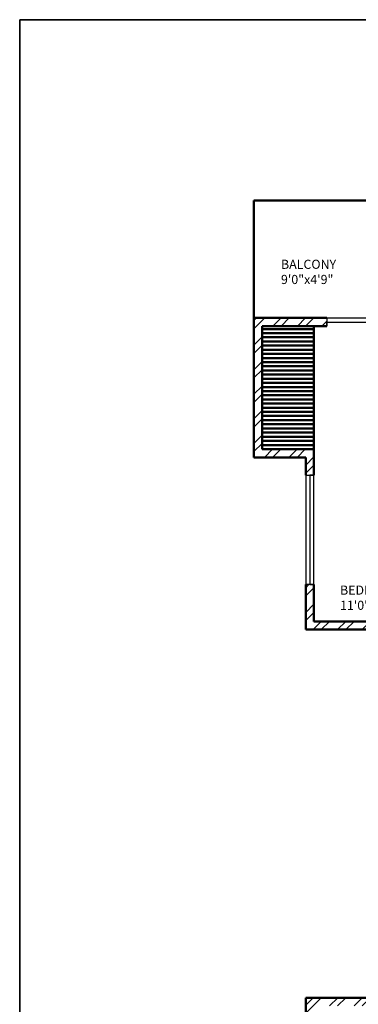
# Model space of a CAD drawing. Units: inches. Extents: x 963 to 2075, y 289 to 2657.
# Tile 59 of 98: x 963 to 1149, y 2117 to 2657. Entities that reach past the tile are written whole.
import ezdxf

# ---------------------------------------------------------------- set-up
doc = ezdxf.new("R2010")
doc.units = ezdxf.units.IN
for name, color, linetype, lineweight in [('A-ANNO-TTLB', 7, 'Continuous', 35), ('A-AREA-IDEN', 7, 'Continuous', 18), ('A-GLAZ', 3, 'Continuous', 25), ('A-WALL', 7, 'Continuous', 50), ('A-WALL-PATT', 8, 'Continuous', 13)]:
    doc.layers.add(name, color=color, linetype=linetype, lineweight=lineweight)
doc.styles.get("Standard").update_dxf_attribs({"font": 'arial.ttf'})

msp = doc.modelspace()

# ---------------------------------------------------------------- hatches: boundary and pattern name
at = {"layer": 'A-WALL-PATT'}
h = msp.add_hatch(dxfattribs=at)
h.set_pattern_fill('ANSI32', color=256)
h.paths.add_polyline_path([(1296.92, 2558.32), (1203.92, 2558.32), (1203.92, 2493.82), (1191.53, 2493.82), (1191.53, 2489.32), (1211.06, 2489.32), (1211.06, 2492.02), (1211.06, 2493.82), (1208.42, 2493.82), (1208.42, 2553.82), (1292.42, 2553.82), (1292.42, 2538.86), (1296.92, 2538.86)])
h.paths.add_polyline_path([(1442.42, 2558.32), (1349.42, 2558.32), (1349.42, 2538.94), (1353.92, 2538.94), (1353.92, 2553.82), (1437.92, 2553.82), (1437.92, 2493.82), (1434.54, 2493.82), (1434.54, 2489.32), (1448.31, 2489.32), (1448.31, 2491.57), (1448.31, 2493.82), (1442.42, 2493.82)])
h.paths.add_polyline_path([(1415.55, 2491.57), (1415.55, 2493.82), (1340.94, 2493.82), (1340.94, 2489.32), (1371.92, 2489.32), (1371.92, 2378.32), (1367.6, 2378.32), (1367.6, 2373.82), (1371.92, 2373.82), (1371.92, 2355.19), (1376.42, 2355.19), (1376.42, 2489.32), (1415.55, 2489.32)])
h.paths.add_polyline_path([(1304.94, 2491.57), (1304.94, 2493.82), (1296.92, 2493.82), (1296.92, 2514.86), (1292.42, 2514.86), (1292.42, 2493.82), (1232.81, 2493.82), (1232.81, 2489.32), (1256.42, 2489.32), (1256.42, 2327.32), (1253.71, 2327.32), (1253.71, 2322.82), (1328.42, 2322.82), (1328.42, 2331.15), (1323.92, 2331.15), (1323.92, 2327.32), (1260.92, 2327.32), (1260.92, 2373.82), (1323.92, 2373.82), (1323.92, 2357.81), (1328.42, 2357.81), (1328.42, 2373.82), (1346.01, 2373.82), (1346.01, 2376.07), (1346.01, 2378.32), (1260.92, 2378.32), (1260.92, 2489.32), (1304.94, 2489.32)])
h.paths.add_polyline_path([(1226.65, 2327.32), (1124.42, 2327.32), (1124.42, 2347.45), (1119.92, 2347.45), (1119.92, 2322.82), (1163.42, 2322.82), (1163.42, 2305.43), (1165.67, 2305.43), (1167.92, 2305.43), (1167.92, 2322.82), (1226.65, 2322.82), (1226.65, 2325.07)])
h.paths.add_polyline_path([(1095.92, 2489.32), (1124.42, 2489.32), (1131.53, 2489.32), (1131.53, 2491.57), (1131.53, 2493.82), (1119.92, 2493.82), (1091.42, 2493.82), (1091.42, 2417.32), (1095.92, 2417.32), (1119.92, 2417.32), (1119.92, 2407.45), (1124.42, 2407.45), (1124.42, 2421.82), (1095.92, 2421.82)])
h.paths.add_polyline_path([(1512.92, 2558.32), (1508.42, 2558.32), (1508.42, 2493.82), (1503.4, 2493.82), (1503.4, 2489.32), (1508.42, 2489.32), (1508.42, 2327.32), (1376.42, 2327.32), (1376.42, 2330.27), (1371.92, 2330.27), (1371.92, 2298.74), (1376.42, 2298.74), (1376.42, 2322.82), (1508.42, 2322.82), (1508.42, 2165.32), (1504.26, 2165.32), (1504.26, 2160.82), (1508.42, 2160.82), (1508.42, 2108.32), (1512.92, 2108.32), (1512.92, 2160.82), (1516.18, 2160.82), (1516.18, 2163.07), (1516.18, 2165.32), (1512.92, 2165.32), (1512.92, 2322.82), (1644.92, 2322.82), (1644.92, 2298.74), (1649.42, 2298.74), (1649.42, 2322.82), (1649.42, 2330.94), (1647.17, 2330.94), (1644.92, 2330.94), (1644.92, 2327.32), (1512.92, 2327.32), (1512.92, 2489.32), (1516.76, 2489.32), (1516.76, 2491.57), (1516.76, 2493.82), (1512.92, 2493.82)])
h.paths.add_polyline_path([(1671.92, 2558.32), (1578.92, 2558.32), (1578.92, 2493.82), (1573.53, 2493.82), (1573.53, 2489.32), (1586.54, 2489.32), (1586.54, 2491.57), (1586.54, 2493.82), (1583.42, 2493.82), (1583.42, 2553.82), (1667.42, 2553.82), (1667.42, 2541.11), (1671.92, 2541.11)])
h.paths.add_polyline_path([(1681.26, 2493.82), (1671.92, 2493.82), (1671.92, 2517.11), (1667.42, 2517.11), (1667.42, 2493.82), (1610.22, 2493.82), (1610.22, 2489.32), (1644.92, 2489.32), (1644.92, 2357.87), (1649.42, 2357.87), (1649.42, 2373.82), (1652.2, 2373.82), (1652.2, 2375.83), (1652.2, 2378.32), (1649.42, 2378.32), (1649.42, 2489.32), (1681.26, 2489.32), (1681.26, 2491.57)])
h.paths.add_polyline_path([(1821.92, 2558.32), (1728.92, 2558.32), (1728.92, 2541), (1733.42, 2541), (1733.42, 2553.82), (1817.42, 2553.82), (1817.42, 2493.82), (1813.51, 2493.82), (1813.51, 2489.32), (1830.08, 2489.32), (1830.08, 2491.57), (1830.08, 2493.82), (1821.92, 2493.82)])
h.paths.add_polyline_path([(1794.24, 2493.82), (1717.26, 2493.82), (1717.26, 2489.32), (1760.42, 2489.32), (1760.42, 2378.32), (1674.4, 2378.32), (1674.4, 2373.82), (1692.92, 2373.82), (1692.92, 2356.95), (1697.42, 2356.95), (1697.42, 2373.82), (1760.42, 2373.82), (1760.42, 2327.32), (1697.42, 2327.32), (1697.42, 2333.34), (1692.92, 2333.34), (1692.92, 2322.82), (1768.04, 2322.82), (1768.04, 2325.07), (1768.04, 2327.32), (1764.92, 2327.32), (1764.92, 2489.32), (1794.24, 2489.32)])
h.paths.add_polyline_path([(1733.42, 2517), (1728.92, 2517), (1728.92, 2493.82), (1733.42, 2493.82)], flags=17)
h.paths.add_polyline_path([(1929.92, 2493.82), (1890.08, 2493.82), (1890.08, 2489.32), (1896.92, 2489.32), (1925.42, 2489.32), (1925.42, 2421.82), (1896.92, 2421.82), (1896.92, 2408.32), (1901.42, 2408.32), (1901.42, 2417.32), (1925.42, 2417.32), (1929.92, 2417.32)])
h.paths.add_polyline_path([(1901.42, 2348.32), (1896.92, 2348.32), (1896.92, 2327.32), (1800.42, 2327.32), (1800.42, 2322.82), (1853.42, 2322.82), (1853.42, 2309.45), (1857.92, 2309.45), (1857.92, 2322.82), (1901.42, 2322.82)])
h.paths.add_polyline_path([(1857.92, 2249.45), (1853.42, 2249.45), (1853.42, 2214.82), (1686.31, 2214.82), (1686.31, 2210.32), (1853.42, 2210.32), (1853.42, 2202.13), (1857.92, 2202.13), (1857.92, 2210.32)])
h.paths.add_polyline_path([(1857.92, 2142.13), (1853.42, 2142.13), (1853.42, 2115.42), (1841.42, 2115.42), (1841.42, 2088.53), (1841.42, 2046.95), (1845.92, 2046.95), (1845.92, 2110.92), (1905.92, 2110.92), (1905.92, 2092.52), (1910.42, 2092.52), (1910.42, 2115.42), (1857.92, 2115.42)])
h.paths.add_polyline_path([(1532.44, 1482.34), (1573.46, 1482.34), (1573.46, 1501), (1532.44, 1501)], flags=9)
h.paths.add_polyline_path([(1438.66, 1486.3), (1479.68, 1486.3), (1479.68, 1504.96), (1438.66, 1504.96)], flags=9)
h.paths.add_polyline_path([(1411.22, 1365.31), (1659.14, 1365.31), (1659.14, 1402.4), (1411.22, 1402.4)], flags=9)
h.paths.add_polyline_path([(1185.67, 2296.3), (1248.16, 2296.3), (1248.16, 2314.95), (1185.67, 2314.95)], flags=9)
h.paths.add_polyline_path([(1177.31, 2187.35), (1216.15, 2187.35), (1216.15, 2206.01), (1177.31, 2206.01)], flags=9)
h.paths.add_polyline_path([(1295.1, 1602.08), (1328.26, 1602.08), (1328.26, 1620.74), (1295.1, 1620.74)], flags=9)
h.paths.add_polyline_path([(1525.13, 2005.99), (1558.39, 2005.99), (1558.39, 2024.65), (1525.13, 2024.65)], flags=9)
h.paths.add_polyline_path([(1459.61, 1977.13), (1472.19, 1977.13), (1472.19, 1987.43), (1459.61, 1987.43)], flags=9)
h.paths.add_polyline_path([(1467.81, 2053.68), (1480.02, 2053.68), (1480.02, 2063.98), (1467.81, 2063.98)], flags=9)
h.paths.add_polyline_path([(1555.18, 2119.02), (1584.56, 2119.02), (1584.56, 2137.68), (1555.18, 2137.68)], flags=25)
h.paths.add_polyline_path([(1405.39, 2115.29), (1444.48, 2115.29), (1444.48, 2133.95), (1405.39, 2133.95)], flags=25)
h.paths.add_polyline_path([(1698.48, 2004.26), (1727.69, 2004.26), (1727.69, 2022.92), (1698.48, 2022.92)], flags=9)
h.paths.add_polyline_path([(1612.16, 1972.86), (1629.02, 1972.86), (1629.02, 1983.16), (1612.16, 1983.16)], flags=9)
h.paths.add_polyline_path([(1608.29, 2060.04), (1625.15, 2060.04), (1625.15, 2070.34), (1608.29, 2070.34)], flags=9)
h.paths.add_polyline_path([(1527.95, 1684.4), (1566.79, 1684.4), (1566.79, 1703.06), (1527.95, 1703.06)], flags=9)
h.paths.add_polyline_path([(1422.79, 1683.59), (1461.63, 1683.59), (1461.63, 1702.25), (1422.79, 1702.25)], flags=9)
h.paths.add_polyline_path([(1531.26, 1732.46), (1574.01, 1732.46), (1574.01, 1751.12), (1531.26, 1751.12)], flags=9)
h.paths.add_polyline_path([(1402.87, 1732.85), (1439.8, 1732.85), (1439.8, 1751.5), (1402.87, 1751.5)], flags=9)
h.paths.add_polyline_path([(1243.12, 1923.13), (1281.96, 1923.13), (1281.96, 1941.79), (1243.12, 1941.79)], flags=9)
h.paths.add_polyline_path([(1181.75, 1792.27), (1244.24, 1792.27), (1244.24, 1810.93), (1181.75, 1810.93)], flags=9)
h.paths.add_polyline_path([(1265.82, 1670.3), (1316.07, 1670.3), (1316.07, 1688.96), (1265.82, 1688.96)], flags=9)
h.paths.add_polyline_path([(1140.26, 1676.05), (1179.1, 1676.05), (1179.1, 1694.71), (1140.26, 1694.71)], flags=9)
h.paths.add_polyline_path([(1107.49, 1490.89), (1143.37, 1490.89), (1143.37, 1509.55), (1107.49, 1509.55)], flags=9)
h.paths.add_polyline_path([(1217.58, 1483.9), (1246.74, 1483.9), (1246.74, 1502.56), (1217.58, 1502.56)], flags=9)
h.paths.add_polyline_path([(1389.21, 1486.92), (1418.37, 1486.92), (1418.37, 1505.58), (1389.21, 1505.58)], flags=9)
h.paths.add_polyline_path([(1672.21, 1602.08), (1705.37, 1602.08), (1705.37, 1620.74), (1672.21, 1620.74)], flags=9)
h.paths.add_polyline_path([(1752.08, 1522.64), (1781.24, 1522.64), (1781.24, 1541.3), (1752.08, 1541.3)], flags=9)
h.paths.add_polyline_path([(1848.27, 1491.26), (1884.16, 1491.26), (1884.16, 1509.92), (1848.27, 1509.92)], flags=9)
h.paths.add_polyline_path([(1822.47, 1685.62), (1861.31, 1685.62), (1861.31, 1704.28), (1822.47, 1704.28)], flags=9)
h.paths.add_polyline_path([(1713.19, 1672.23), (1763.44, 1672.23), (1763.44, 1690.89), (1713.19, 1690.89)], flags=9)
h.paths.add_polyline_path([(1736.62, 1790.58), (1799.11, 1790.58), (1799.11, 1809.24), (1736.62, 1809.24)], flags=9)
h.paths.add_polyline_path([(1691.49, 1916.36), (1730.33, 1916.36), (1730.33, 1935.01), (1691.49, 1935.01)], flags=9)
h.paths.add_polyline_path([(1764.87, 1973.92), (1794.31, 1973.92), (1794.31, 1992.58), (1764.87, 1992.58)], flags=9)
h.paths.add_polyline_path([(1767.85, 2034.02), (1797.29, 2034.02), (1797.29, 2052.67), (1767.85, 2052.67)], flags=9)
h.paths.add_polyline_path([(1851.59, 2060.33), (1880.75, 2060.33), (1880.75, 2078.99), (1851.59, 2078.99)], flags=25)
h.paths.add_polyline_path([(1688.49, 2086.87), (1727.33, 2086.87), (1727.33, 2105.53), (1688.49, 2105.53)], flags=9)
h.paths.add_polyline_path([(1537.74, 2293.58), (1580.49, 2293.58), (1580.49, 2312.24), (1537.74, 2312.24)], flags=25)
h.paths.add_polyline_path([(1425.59, 2296.11), (1468.34, 2296.11), (1468.34, 2314.77), (1425.59, 2314.77)], flags=25)
h.paths.add_polyline_path([(1278.52, 2004.18), (1307.72, 2004.18), (1307.72, 2022.84), (1278.52, 2022.84)], flags=9)
h.paths.add_polyline_path([(1193.28, 1973.63), (1222.72, 1973.63), (1222.72, 1992.29), (1193.28, 1992.29)], flags=9)
h.paths.add_polyline_path([(1192.41, 2040.58), (1221.84, 2040.58), (1221.84, 2059.23), (1192.41, 2059.23)], flags=9)
h.paths.add_polyline_path([(1130.6, 1951.39), (1159.76, 1951.39), (1159.76, 1970.05), (1130.6, 1970.05)], flags=9)
h.paths.add_polyline_path([(1132.83, 2052.49), (1161.98, 2052.49), (1161.98, 2071.15), (1132.83, 2071.15)], flags=9)
h.paths.add_polyline_path([(1265.13, 2334.62), (1315.38, 2334.62), (1315.38, 2353.28), (1265.13, 2353.28)], flags=25)
h.paths.add_polyline_path([(1136.74, 2330.79), (1175.58, 2330.79), (1175.58, 2349.44), (1136.74, 2349.44)], flags=9)
h.paths.add_polyline_path([(1287.42, 2417.2), (1320.58, 2417.2), (1320.58, 2435.86), (1287.42, 2435.86)], flags=25)
h.paths.add_polyline_path([(1430.99, 2329.16), (1469.83, 2329.16), (1469.83, 2347.82), (1430.99, 2347.82)], flags=25)
h.paths.add_polyline_path([(1525.42, 2329.21), (1564.26, 2329.21), (1564.26, 2347.87), (1525.42, 2347.87)], flags=25)
h.paths.add_polyline_path([(1684.52, 2382.8), (1717.68, 2382.8), (1717.68, 2401.46), (1684.52, 2401.46)], flags=25)
h.paths.add_polyline_path([(1704.81, 2340.29), (1755.05, 2340.29), (1755.05, 2358.95), (1704.81, 2358.95)], flags=25)
h.paths.add_polyline_path([(1694.11, 2287.76), (1756.6, 2287.76), (1756.6, 2306.41), (1694.11, 2306.41)], flags=9)
h.paths.add_polyline_path([(1815.78, 2329.86), (1854.62, 2329.86), (1854.62, 2348.52), (1815.78, 2348.52)], flags=9)
h.paths.add_polyline_path([(1842.87, 2514.26), (1878.76, 2514.26), (1878.76, 2532.91), (1842.87, 2532.91)], flags=9)
h.paths.add_polyline_path([(1769.51, 2531.45), (1798.67, 2531.45), (1798.67, 2550.1), (1769.51, 2550.1)], flags=25)
h.paths.add_polyline_path([(1594.77, 2518.47), (1623.93, 2518.47), (1623.93, 2537.13), (1594.77, 2537.13)], flags=25)
h.paths.add_polyline_path([(1520.72, 2516.18), (1556.61, 2516.18), (1556.61, 2534.84), (1520.72, 2534.84)], flags=25)
h.paths.add_polyline_path([(1464.46, 2516.69), (1500.34, 2516.69), (1500.34, 2535.35), (1464.46, 2535.35)], flags=25)
h.paths.add_polyline_path([(1365.7, 2528.97), (1394.85, 2528.97), (1394.85, 2547.63), (1365.7, 2547.63)], flags=25)
h.paths.add_polyline_path([(1222.84, 2516.23), (1252, 2516.23), (1252, 2534.89), (1222.84, 2534.89)], flags=25)
h.paths.add_polyline_path([(1104.55, 2509.6), (1140.43, 2509.6), (1140.43, 2528.26), (1104.55, 2528.26)], flags=9)
h = msp.add_hatch(dxfattribs=at)
h.set_pattern_fill('ANSI32', color=256)
h.paths.add_polyline_path([(1335.97, 2212.57), (1335.97, 2214.82), (1167.92, 2214.82), (1167.92, 2245.43), (1163.42, 2245.43), (1163.42, 2210.32), (1163.42, 2194.81), (1167.92, 2194.81), (1167.92, 2210.32), (1335.97, 2210.32)])
h.paths.add_polyline_path([(1532.44, 1482.34), (1573.46, 1482.34), (1573.46, 1501), (1532.44, 1501)], flags=9)
h.paths.add_polyline_path([(1438.66, 1486.3), (1479.68, 1486.3), (1479.68, 1504.96), (1438.66, 1504.96)], flags=9)
h.paths.add_polyline_path([(1411.22, 1365.31), (1659.14, 1365.31), (1659.14, 1402.4), (1411.22, 1402.4)], flags=9)
h.paths.add_polyline_path([(1185.67, 2296.3), (1248.16, 2296.3), (1248.16, 2314.95), (1185.67, 2314.95)], flags=9)
h.paths.add_polyline_path([(1177.31, 2187.35), (1216.15, 2187.35), (1216.15, 2206.01), (1177.31, 2206.01)], flags=9)
h.paths.add_polyline_path([(1295.1, 1602.08), (1328.26, 1602.08), (1328.26, 1620.74), (1295.1, 1620.74)], flags=9)
h.paths.add_polyline_path([(1525.13, 2005.99), (1558.39, 2005.99), (1558.39, 2024.65), (1525.13, 2024.65)], flags=9)
h.paths.add_polyline_path([(1459.61, 1977.13), (1472.19, 1977.13), (1472.19, 1987.43), (1459.61, 1987.43)], flags=9)
h.paths.add_polyline_path([(1467.81, 2053.68), (1480.02, 2053.68), (1480.02, 2063.98), (1467.81, 2063.98)], flags=9)
h.paths.add_polyline_path([(1555.18, 2119.02), (1584.56, 2119.02), (1584.56, 2137.68), (1555.18, 2137.68)], flags=9)
h.paths.add_polyline_path([(1405.39, 2115.29), (1444.48, 2115.29), (1444.48, 2133.95), (1405.39, 2133.95)], flags=9)
h.paths.add_polyline_path([(1698.48, 2004.26), (1727.69, 2004.26), (1727.69, 2022.92), (1698.48, 2022.92)], flags=9)
h.paths.add_polyline_path([(1612.16, 1972.86), (1629.02, 1972.86), (1629.02, 1983.16), (1612.16, 1983.16)], flags=9)
h.paths.add_polyline_path([(1608.29, 2060.04), (1625.15, 2060.04), (1625.15, 2070.34), (1608.29, 2070.34)], flags=9)
h.paths.add_polyline_path([(1527.95, 1684.4), (1566.79, 1684.4), (1566.79, 1703.06), (1527.95, 1703.06)], flags=9)
h.paths.add_polyline_path([(1422.79, 1683.59), (1461.63, 1683.59), (1461.63, 1702.25), (1422.79, 1702.25)], flags=9)
h.paths.add_polyline_path([(1531.26, 1732.46), (1574.01, 1732.46), (1574.01, 1751.12), (1531.26, 1751.12)], flags=9)
h.paths.add_polyline_path([(1402.87, 1732.85), (1439.8, 1732.85), (1439.8, 1751.5), (1402.87, 1751.5)], flags=9)
h.paths.add_polyline_path([(1243.12, 1923.13), (1281.96, 1923.13), (1281.96, 1941.79), (1243.12, 1941.79)], flags=9)
h.paths.add_polyline_path([(1181.75, 1792.27), (1244.24, 1792.27), (1244.24, 1810.93), (1181.75, 1810.93)], flags=9)
h.paths.add_polyline_path([(1265.82, 1670.3), (1316.07, 1670.3), (1316.07, 1688.96), (1265.82, 1688.96)], flags=9)
h.paths.add_polyline_path([(1140.26, 1676.05), (1179.1, 1676.05), (1179.1, 1694.71), (1140.26, 1694.71)], flags=9)
h.paths.add_polyline_path([(1107.49, 1490.89), (1143.37, 1490.89), (1143.37, 1509.55), (1107.49, 1509.55)], flags=9)
h.paths.add_polyline_path([(1217.58, 1483.9), (1246.74, 1483.9), (1246.74, 1502.56), (1217.58, 1502.56)], flags=9)
h.paths.add_polyline_path([(1389.21, 1486.92), (1418.37, 1486.92), (1418.37, 1505.58), (1389.21, 1505.58)], flags=9)
h.paths.add_polyline_path([(1672.21, 1602.08), (1705.37, 1602.08), (1705.37, 1620.74), (1672.21, 1620.74)], flags=9)
h.paths.add_polyline_path([(1752.08, 1522.64), (1781.24, 1522.64), (1781.24, 1541.3), (1752.08, 1541.3)], flags=9)
h.paths.add_polyline_path([(1848.27, 1491.26), (1884.16, 1491.26), (1884.16, 1509.92), (1848.27, 1509.92)], flags=9)
h.paths.add_polyline_path([(1822.47, 1685.62), (1861.31, 1685.62), (1861.31, 1704.28), (1822.47, 1704.28)], flags=9)
h.paths.add_polyline_path([(1713.19, 1672.23), (1763.44, 1672.23), (1763.44, 1690.89), (1713.19, 1690.89)], flags=9)
h.paths.add_polyline_path([(1736.62, 1790.58), (1799.11, 1790.58), (1799.11, 1809.24), (1736.62, 1809.24)], flags=9)
h.paths.add_polyline_path([(1691.49, 1916.36), (1730.33, 1916.36), (1730.33, 1935.01), (1691.49, 1935.01)], flags=9)
h.paths.add_polyline_path([(1764.87, 1973.92), (1794.31, 1973.92), (1794.31, 1992.58), (1764.87, 1992.58)], flags=9)
h.paths.add_polyline_path([(1767.85, 2034.02), (1797.29, 2034.02), (1797.29, 2052.67), (1767.85, 2052.67)], flags=9)
h.paths.add_polyline_path([(1851.59, 2060.33), (1880.75, 2060.33), (1880.75, 2078.99), (1851.59, 2078.99)], flags=9)
h.paths.add_polyline_path([(1688.49, 2086.87), (1727.33, 2086.87), (1727.33, 2105.53), (1688.49, 2105.53)], flags=9)
h.paths.add_polyline_path([(1537.74, 2293.58), (1580.49, 2293.58), (1580.49, 2312.24), (1537.74, 2312.24)], flags=9)
h.paths.add_polyline_path([(1425.59, 2296.11), (1468.34, 2296.11), (1468.34, 2314.77), (1425.59, 2314.77)], flags=9)
h.paths.add_polyline_path([(1278.52, 2004.18), (1307.72, 2004.18), (1307.72, 2022.84), (1278.52, 2022.84)], flags=9)
h.paths.add_polyline_path([(1193.28, 1973.63), (1222.72, 1973.63), (1222.72, 1992.29), (1193.28, 1992.29)], flags=9)
h.paths.add_polyline_path([(1192.41, 2040.58), (1221.84, 2040.58), (1221.84, 2059.23), (1192.41, 2059.23)], flags=9)
h.paths.add_polyline_path([(1130.6, 1951.39), (1159.76, 1951.39), (1159.76, 1970.05), (1130.6, 1970.05)], flags=9)
h.paths.add_polyline_path([(1132.83, 2052.49), (1161.98, 2052.49), (1161.98, 2071.15), (1132.83, 2071.15)], flags=9)
h.paths.add_polyline_path([(1265.13, 2334.62), (1315.38, 2334.62), (1315.38, 2353.28), (1265.13, 2353.28)], flags=9)
h.paths.add_polyline_path([(1136.74, 2330.79), (1175.58, 2330.79), (1175.58, 2349.44), (1136.74, 2349.44)], flags=9)
h.paths.add_polyline_path([(1287.42, 2417.2), (1320.58, 2417.2), (1320.58, 2435.86), (1287.42, 2435.86)], flags=9)
h.paths.add_polyline_path([(1430.99, 2329.16), (1469.83, 2329.16), (1469.83, 2347.82), (1430.99, 2347.82)], flags=9)
h.paths.add_polyline_path([(1525.42, 2329.21), (1564.26, 2329.21), (1564.26, 2347.87), (1525.42, 2347.87)], flags=9)
h.paths.add_polyline_path([(1684.52, 2382.8), (1717.68, 2382.8), (1717.68, 2401.46), (1684.52, 2401.46)], flags=9)
h.paths.add_polyline_path([(1704.81, 2340.29), (1755.05, 2340.29), (1755.05, 2358.95), (1704.81, 2358.95)], flags=9)
h.paths.add_polyline_path([(1694.11, 2287.76), (1756.6, 2287.76), (1756.6, 2306.41), (1694.11, 2306.41)], flags=9)
h.paths.add_polyline_path([(1815.78, 2329.86), (1854.62, 2329.86), (1854.62, 2348.52), (1815.78, 2348.52)], flags=9)
h.paths.add_polyline_path([(1842.87, 2514.26), (1878.76, 2514.26), (1878.76, 2532.91), (1842.87, 2532.91)], flags=9)
h.paths.add_polyline_path([(1769.51, 2531.45), (1798.67, 2531.45), (1798.67, 2550.1), (1769.51, 2550.1)], flags=9)
h.paths.add_polyline_path([(1594.77, 2518.47), (1623.93, 2518.47), (1623.93, 2537.13), (1594.77, 2537.13)], flags=9)
h.paths.add_polyline_path([(1520.72, 2516.18), (1556.61, 2516.18), (1556.61, 2534.84), (1520.72, 2534.84)], flags=9)
h.paths.add_polyline_path([(1464.46, 2516.69), (1500.34, 2516.69), (1500.34, 2535.35), (1464.46, 2535.35)], flags=9)
h.paths.add_polyline_path([(1365.7, 2528.97), (1394.85, 2528.97), (1394.85, 2547.63), (1365.7, 2547.63)], flags=9)
h.paths.add_polyline_path([(1222.84, 2516.23), (1252, 2516.23), (1252, 2534.89), (1222.84, 2534.89)], flags=9)
h.paths.add_polyline_path([(1104.55, 2509.6), (1140.43, 2509.6), (1140.43, 2528.26), (1104.55, 2528.26)], flags=9)
h = msp.add_hatch(dxfattribs=at)
h.set_pattern_fill('ANSI32', color=256)
h.paths.add_polyline_path([(1473.61, 2163.07), (1473.61, 2165.32), (1376.42, 2165.32), (1376.42, 2227.98), (1371.92, 2227.98), (1371.92, 2214.82), (1368.41, 2214.82), (1368.41, 2210.32), (1371.92, 2210.32), (1371.92, 2160.82), (1395.92, 2160.82), (1395.92, 2090.32), (1217.34, 2090.32), (1217.34, 2085.82), (1395.92, 2085.82), (1458.92, 2085.82), (1458.92, 2108.32), (1454.42, 2108.32), (1454.42, 2090.32), (1400.42, 2090.32), (1400.42, 2160.82), (1473.61, 2160.82)])
h.paths.add_polyline_path([(1649.42, 2210.32), (1653.23, 2210.32), (1653.23, 2214.82), (1649.42, 2214.82), (1649.42, 2227.98), (1644.92, 2227.98), (1644.92, 2165.32), (1550.1, 2165.32), (1550.1, 2160.82), (1620.92, 2160.82), (1620.92, 2112.82), (1555.45, 2112.82), (1555.45, 2108.32), (1584.33, 2108.32), (1584.33, 2084.92), (1588.83, 2084.92), (1588.83, 2108.32), (1625.42, 2108.32), (1667.95, 2108.32), (1667.95, 2022.67), (1588.83, 2022.67), (1588.83, 2047.41), (1584.33, 2047.41), (1584.33, 1996), (1588.83, 1996), (1588.83, 2018.32), (1667.95, 2018.17), (1667.95, 1928.32), (1625.42, 1928.32), (1625.42, 1923.82), (1672.45, 1923.82), (1672.45, 1928.32), (1672.45, 1946.66), (1785.45, 1946.66), (1785.45, 1951.16), (1743.03, 1951.16), (1743.03, 2017.92), (1841.42, 2017.92), (1841.42, 2014.77), (1845.92, 2014.77), (1845.92, 2017.92), (1905.92, 2017.92), (1905.92, 1987.51), (1910.42, 1987.51), (1910.42, 2022.42), (1910.42, 2068.52), (1905.92, 2068.52), (1905.92, 2022.42), (1845.92, 2022.42), (1845.92, 2025.85), (1843.67, 2025.85), (1841.42, 2025.85), (1841.42, 2022.42), (1743.03, 2022.42), (1743.03, 2084.03), (1768.45, 2084.03), (1785.45, 2084.03), (1785.45, 2088.53), (1672.45, 2088.53), (1672.45, 2112.82), (1667.95, 2112.82), (1625.42, 2112.82), (1625.42, 2160.82), (1649.42, 2160.82)])
h.paths.add_polyline_path([(1672.45, 2084.03), (1738.53, 2084.03), (1738.53, 1951.16), (1672.45, 1951.16)], flags=16)
h.paths.add_polyline_path([(1672.45, 2084.03), (1738.53, 2084.03), (1705.49, 2017.6)], flags=0)
h.paths.add_polyline_path([(1262.77, 2085.82), (1258.27, 2085.82), (1258.27, 2023.28), (1184.42, 2023.28), (1184.42, 2018.78), (1258.27, 2018.78), (1258.27, 1950.82), (1262.77, 1950.82)])
h.paths.add_polyline_path([(1312.27, 2085.82), (1307.77, 2085.82), (1307.77, 1950.82), (1312.27, 1950.82)])
h.paths.add_polyline_path([(1458.92, 1950.82), (1395.92, 1950.82), (1216.57, 1950.82), (1216.57, 1946.32), (1346.42, 1946.32), (1395.92, 1946.32), (1395.92, 1875.82), (1371.92, 1875.82), (1371.92, 1826.32), (1368.93, 1826.32), (1368.93, 1821.82), (1371.92, 1821.82), (1371.92, 1813.62), (1376.42, 1813.62), (1376.42, 1871.32), (1474.5, 1871.32), (1474.5, 1873.57), (1474.5, 1875.82), (1400.42, 1875.82), (1400.42, 1946.32), (1454.42, 1946.32), (1454.42, 1928.32), (1458.92, 1928.32)])
h.paths.add_polyline_path([(1184.42, 2120.78), (1167.92, 2120.78), (1167.92, 2134.81), (1165.67, 2134.81), (1163.42, 2134.81), (1163.42, 2120.78), (1119.92, 2120.78), (1119.92, 2098.1), (1124.42, 2098.1), (1124.42, 2116.28), (1167.92, 2116.28), (1179.92, 2116.28), (1179.92, 2045.92), (1184.42, 2045.92), (1184.42, 2090.32), (1184.42, 2116.28)])
h.paths.add_polyline_path([(1124.42, 2018.78), (1179.92, 2018.78), (1179.92, 2016.29), (1184.42, 2016.29), (1184.42, 2023.28), (1184.42, 2026.59), (1182.17, 2026.59), (1179.92, 2026.59), (1179.92, 2023.28), (1124.42, 2023.28), (1124.42, 2074.1), (1119.92, 2074.1), (1119.92, 2018.78), (1119.92, 1979.63), (1124.42, 1979.63)])
h.paths.add_polyline_path([(1184.42, 1925.78), (1184.42, 1946.32), (1184.42, 1996.07), (1182.17, 1996.07), (1179.92, 1996.07), (1179.92, 1925.78), (1124.42, 1925.78), (1124.42, 1955.63), (1119.92, 1955.5), (1119.92, 1921.28), (1158.92, 1921.28), (1158.92, 1909.98), (1163.42, 1909.98), (1163.42, 1921.28), (1184.42, 1921.28)])
h.paths.add_polyline_path([(1341.45, 1826.32), (1163.42, 1826.32), (1163.42, 1849.98), (1158.92, 1849.98), (1158.92, 1821.82), (1158.92, 1804.03), (1163.42, 1804.03), (1163.42, 1821.82), (1341.45, 1821.82)])
h.paths.add_polyline_path([(1222.98, 1713.82), (1163.42, 1713.82), (1163.42, 1744.03), (1161.17, 1744.03), (1158.92, 1744.03), (1158.92, 1713.82), (1119.92, 1713.82), (1119.92, 1694.65), (1124.42, 1694.65), (1124.42, 1709.32), (1158.92, 1709.32), (1222.98, 1709.32)])
h.paths.add_polyline_path([(1328.42, 1713.82), (1252.04, 1713.82), (1252.04, 1711.57), (1252.04, 1709.32), (1256.42, 1709.32), (1256.42, 1547.32), (1232.94, 1547.32), (1232.94, 1545.07), (1232.94, 1542.82), (1292.42, 1542.82), (1292.42, 1527.63), (1296.92, 1527.63), (1296.92, 1542.82), (1299.46, 1542.82), (1299.46, 1547.32), (1260.92, 1547.32), (1260.92, 1658.32), (1343.66, 1658.32), (1343.66, 1660.57), (1343.66, 1662.82), (1328.42, 1662.82), (1328.42, 1676.59), (1327.4, 1676.59), (1323.92, 1676.59), (1323.92, 1662.82), (1260.92, 1662.82), (1260.92, 1709.32), (1323.92, 1709.32), (1323.92, 1699.85), (1328.42, 1699.85)])
h.paths.add_polyline_path([(1649.42, 1875.82), (1625.42, 1875.82), (1625.42, 1928.32), (1620.92, 1928.32), (1588.83, 1928.32), (1588.83, 1950.59), (1584.33, 1950.59), (1584.33, 1928.32), (1555.45, 1928.32), (1555.45, 1923.82), (1620.92, 1923.82), (1620.92, 1875.82), (1548.95, 1875.82), (1548.95, 1873.57), (1548.95, 1871.32), (1644.92, 1871.32), (1644.92, 1813.62), (1649.42, 1813.62), (1649.42, 1821.82), (1652.04, 1821.82), (1652.04, 1824.07), (1652.04, 1826.32), (1649.42, 1826.32)])
h.paths.add_polyline_path([(1512.92, 1871.32), (1516.48, 1871.32), (1516.48, 1875.82), (1512.92, 1875.82), (1512.92, 1923.82), (1512.92, 1928.32), (1512.92, 1930.83), (1508.42, 1930.83), (1508.42, 1875.82), (1504.41, 1875.82), (1504.41, 1871.32), (1508.42, 1871.32), (1508.42, 1713.82), (1376.42, 1713.82), (1376.42, 1743.32), (1371.92, 1743.32), (1371.92, 1709.32), (1371.92, 1706.01), (1376.42, 1706.01), (1376.42, 1709.32), (1508.42, 1709.32), (1508.42, 1547.32), (1501.87, 1547.32), (1501.87, 1542.82), (1508.42, 1542.82), (1508.42, 1482.82), (1508.42, 1436.32), (1512.92, 1436.32), (1512.92, 1542.82), (1519.32, 1542.82), (1519.32, 1545.07), (1519.32, 1547.32), (1512.92, 1547.32), (1512.92, 1709.32), (1644.92, 1709.32), (1644.92, 1707.55), (1649.42, 1707.55), (1649.42, 1709.32), (1649.42, 1743.32), (1644.92, 1743.32), (1644.92, 1713.82), (1512.92, 1713.82)])
h.paths.add_polyline_path([(1129.88, 1545.07), (1129.88, 1547.32), (1124.42, 1547.32), (1095.92, 1547.32), (1095.92, 1614.82), (1124.42, 1614.82), (1124.42, 1619.32), (1095.92, 1619.32), (1091.42, 1619.32), (1091.42, 1542.82), (1095.92, 1542.82), (1119.92, 1542.82), (1129.88, 1542.82)])
h.paths.add_polyline_path([(1208.42, 1542.82), (1211.74, 1542.82), (1211.74, 1547.32), (1198.85, 1547.32), (1198.85, 1542.82), (1203.92, 1542.82), (1203.92, 1478.32), (1208.42, 1478.32), (1296.92, 1478.32), (1296.92, 1503.63), (1292.42, 1503.63), (1292.42, 1482.82), (1208.42, 1482.82)])
h.paths.add_polyline_path([(1430.42, 1542.82), (1435.7, 1542.82), (1435.7, 1545.07), (1435.7, 1547.32), (1422.66, 1547.32), (1422.66, 1545.07), (1422.66, 1542.82), (1425.92, 1542.82), (1425.92, 1482.86), (1341.92, 1482.86), (1341.92, 1502.73), (1337.42, 1502.73), (1337.42, 1478.36), (1425.92, 1478.36), (1425.92, 1440.82), (1425.92, 1436.32), (1430.42, 1436.32)])
h.paths.add_polyline_path([(1698.48, 2004.26), (1727.69, 2004.26), (1727.69, 2022.92), (1698.48, 2022.92)], flags=8)

# ---------------------------------------------------------------- linework, layer by layer
at = {"layer": 'A-ANNO-TTLB'}
msp.add_lwpolyline([(962.81, 2657.49), (2074.6, 2657.49), (2074.6, 1303.08), (962.81, 1303.08)], close=True, dxfattribs=at)
at = {"layer": 'A-GLAZ'}
for p, q in [((1131.53, 2493.82), (1131.53, 2489.32)), ((1131.53, 2493.82), (1173.74, 2493.82)), ((1131.53, 2489.32), (1131.53, 2491.57)), ((1131.53, 2491.57), (1131.53, 2491.57)), ((1131.53, 2491.57), (1191.53, 2491.57)), ((1119.92, 2407.45), (1124.42, 2407.45)), ((1119.92, 2407.45), (1119.92, 2347.45)), ((1124.42, 2407.45), (1122.17, 2407.45)), ((1122.17, 2407.45), (1122.17, 2347.45)), ((1124.42, 2347.45), (1124.42, 2407.45)), ((1124.42, 2347.45), (1119.92, 2347.45)), ((1122.17, 2347.45), (1124.42, 2347.45))]:
    msp.add_line(p, q, dxfattribs=at)
at = {"layer": 'A-WALL'}
for p, q in [((1296.92, 2558.32), (1091.42, 2558.32)), ((1091.42, 2558.32), (1091.42, 2553.82)), ((1091.42, 2493.82), (1091.42, 2553.82)), ((1119.92, 2493.82), (1091.42, 2493.82)), ((1091.42, 2417.32), (1091.42, 2493.82)), ((1119.92, 2493.82), (1131.53, 2493.82)), ((1095.92, 2489.32), (1095.92, 2421.82)), ((1124.42, 2489.32), (1095.92, 2489.32)), ((1124.42, 2487.75), (1095.92, 2487.75)), ((1124.42, 2489.32), (1131.53, 2489.32)), ((1124.42, 2489.32), (1124.42, 2407.45)), ((1124.42, 2485.48), (1095.92, 2485.48)), ((1124.42, 2483.2), (1095.92, 2483.2)), ((1124.42, 2480.93), (1095.92, 2480.93)), ((1124.42, 2478.66), (1095.92, 2478.66)), ((1124.42, 2476.38), (1095.92, 2476.38)), ((1124.42, 2474.11), (1095.92, 2474.11)), ((1124.42, 2471.83), (1095.92, 2471.83)), ((1124.42, 2469.56), (1095.92, 2469.56)), ((1124.42, 2467.29), (1095.92, 2467.29)), ((1124.42, 2465.01), (1095.92, 2465.01)), ((1124.42, 2462.74), (1095.92, 2462.74)), ((1124.42, 2460.47), (1095.92, 2460.47)), ((1124.42, 2458.19), (1095.92, 2458.19)), ((1124.42, 2455.92), (1095.92, 2455.92)), ((1124.42, 2453.65), (1095.92, 2453.65)), ((1124.42, 2451.37), (1095.92, 2451.37)), ((1124.42, 2449.1), (1095.92, 2449.1)), ((1124.42, 2446.83), (1095.92, 2446.83)), ((1124.42, 2444.55), (1095.92, 2444.55)), ((1124.42, 2442.28), (1095.92, 2442.28)), ((1124.42, 2440.01), (1095.92, 2440.01)), ((1124.42, 2437.73), (1095.92, 2437.73)), ((1124.42, 2435.46), (1095.92, 2435.46)), ((1124.42, 2433.19), (1095.92, 2433.19)), ((1124.42, 2430.91), (1095.92, 2430.91)), ((1124.42, 2428.64), (1095.92, 2428.64)), ((1124.42, 2426.36), (1095.92, 2426.36)), ((1124.42, 2424.09), (1095.92, 2424.09)), ((1095.92, 2421.82), (1124.42, 2421.82)), ((1124.42, 2421.82), (1095.92, 2421.82)), ((1124.42, 2421.82), (1124.42, 2417.32)), ((1095.92, 2417.32), (1091.42, 2417.32)), ((1119.92, 2417.32), (1095.92, 2417.32)), ((1119.92, 2417.32), (1119.92, 2407.45)), ((1119.92, 2347.45), (1119.92, 2322.82)), ((1124.42, 2347.45), (1124.42, 2327.32)), ((1124.42, 2327.32), (1227.75, 2327.32)), ((1119.92, 2322.82), (1163.42, 2322.82)), ((1119.92, 2120.78), (1119.92, 2098.1)), ((1163.42, 2120.78), (1119.92, 2120.78))]:
    msp.add_line(p, q, dxfattribs=at)

# ---------------------------------------------------------------- texts
at = {"layer": 'A-AREA-IDEN', "char_height": 5, "attachment_point": 1}
for s, width, insert in [('BALCONY\\P9\'0"x4\'9"', 197.4141, (1106.31, 2525.77)), ('BEDROOM\\P11\'0"x13\'6"', 128.4596, (1138.75, 2346.96))]:
    msp.add_mtext_dynamic_manual_height_columns(s, width=width, gutter_width=12.5, heights=[0], dxfattribs=dict(at, insert=insert))

doc.saveas('drawing.dxf')
